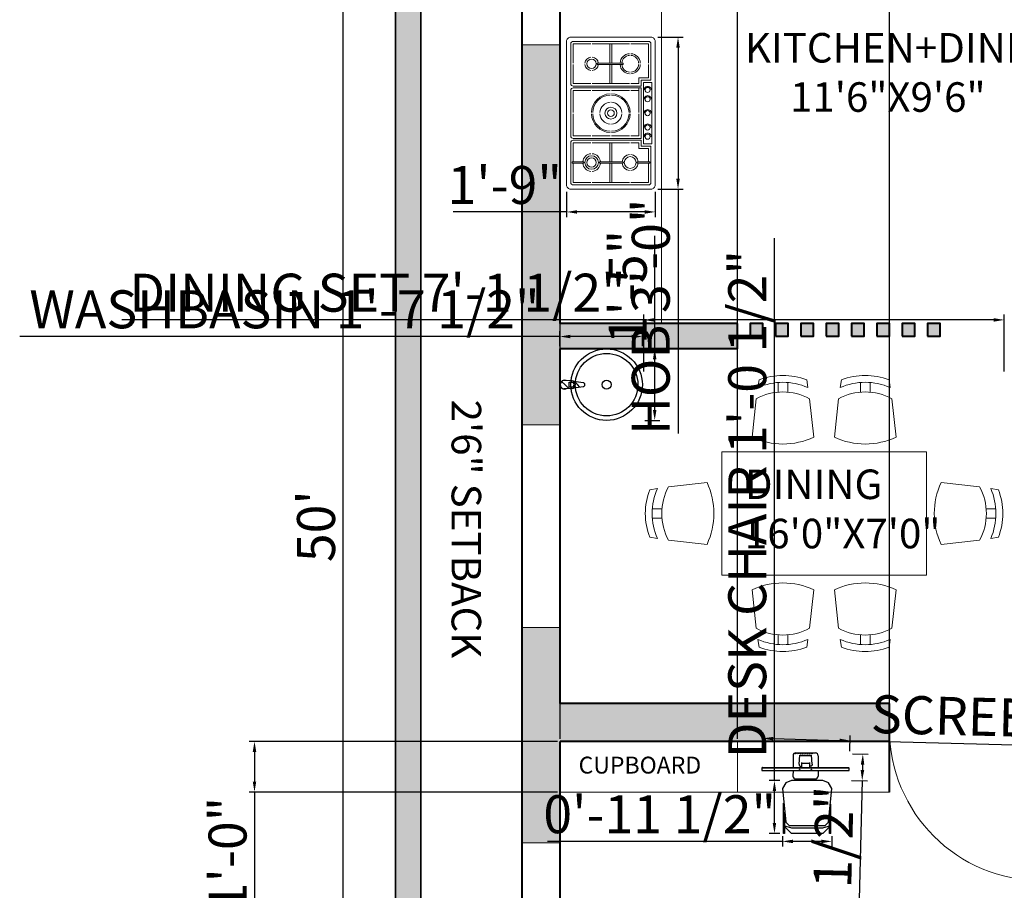
# Model space of a CAD drawing. Units: inches. Extents: x 2337 to 3570, y 1258 to 1938.
# Tile 3 of 30: x 2337 to 2570, y 1507 to 1713. Entities that reach past the tile are written whole.
import ezdxf

# ---------------------------------------------------------------- set-up
doc = ezdxf.new("R2010")
doc.units = ezdxf.units.IN
for name, color, linetype, lineweight in [('A-ANNO-DIMS', 2, 'Continuous', 18), ('A-ANNO-TEXT', 7, 'Continuous', 18), ('A-AREA-IDEN', 7, 'Continuous', 18), ('A-DOOR', 4, 'Continuous', 20), ('A-EQPM', 9, 'Continuous', 18), ('A-FLOR-CASE', 34, 'Continuous', 18), ('A-GLAZ', 4, 'Continuous', 18), ('A-WALL', 7, 'Continuous', 40), ('C-PROP', 7, 'Continuous', 35), ('furn', 8, 'Continuous', 18), ('Сантехника', 9, 'Continuous', 18)]:
    doc.layers.add(name, color=color, linetype=linetype, lineweight=lineweight)
doc.layers.add('A-WALL-PATT', color=18, linetype='Continuous', lineweight=13, true_color=0x000000)
doc.layers.add('C-PROP-PATT', color=251, linetype='Continuous', lineweight=13, true_color=0x636466)
for name, color, linetype in [('NOITHAT', 21, 'Continuous'), ('SANTEH', 7, 'Continuous'), ('window', 130, 'Continuous')]:
    doc.layers.add(name, color=color, linetype=linetype)
doc.styles.get("Standard").update_dxf_attribs({"font": 'arial.ttf'})
doc.dimstyles.new('ISO-25', dxfattribs={"dimtxt": 9, "dimasz": 2.5, "dimexe": 1.25, "dimexo": 0.625, "dimtad": 1, "dimdec": 1, "dimlunit": 3, "dimtxsty": 'Standard', "dimcen": 2.5, "dimadec": 0, "dimazin": 0, "dimtfac": 1, "dimtdec": 1, "dimtmove": 0, "dimatfit": 3, "dimfxl": 1, "dimarcsym": 0})
pattern_1 = [(45, (-0.056, -259.036), (-35.355, 35.355), [])]

# ---------------------------------------------------------------- blocks, each defined once
blk = doc.blocks.new('*U2')
for p, q in [((0, 0), (0, -6)), ((36, 0), (36, -6))]:
    blk.add_line(p, q)
blk.add_lwpolyline([(0, 0), (0, 36), (1.75, 36), (1.75, 0)], close=True)
blk.add_arc((0, 0), 36, 0, 90)
blk = doc.blocks.new('*D7')
at = {"layer": 'A-ANNO-DIMS', "color": 0, "lineweight": -2, "transparency": 16777216}
for p, q in [((2425.21, 1893.12), (2412.15, 1893.12)), ((2413.4, 1890.62), (2413.4, 1295.62)), ((2425.21, 1293.12), (2412.15, 1293.12))]:
    blk.add_line(p, q, dxfattribs=at)
at = {"layer": 'A-ANNO-DIMS', "color": 0, "transparency": 16777216}
for points in [[(2412.98, 1890.62), (2413.81, 1890.62), (2413.4, 1893.12)], [(2412.98, 1295.62), (2413.81, 1295.62), (2413.4, 1293.12)]]:
    blk.add_solid(points, dxfattribs=at)
at = {"layer": 'Defpoints', "color": 0, "transparency": 16777216}
for p in [(2425.84, 1893.12), (2413.4, 1293.12), (2425.84, 1293.12)]:
    blk.add_point(p, dxfattribs=at)
at = {"layer": 'A-ANNO-DIMS', "color": 0, "transparency": 16777216, "insert": (2408.18, 1593.12), "char_height": 9, "attachment_point": 5, "rotation": 90}
blk.add_mtext("50'", dxfattribs=at)
blk = doc.blocks.new('table-23')
at = {"color": 0, "linetype": 'ByBlock'}
for p, q in [((-0.6323, 0.4685), (-0.6236, 0.5245)), ((-0.485, 0.5057), (-0.485, 0.4355)), ((-0.415, 0.5057), (-0.415, 0.4355)), ((-0.2677, 0.4685), (-0.2764, 0.5245)), ((-0.675, 0.107), (-0.645, 0.387)), ((-0.225, 0.107), (-0.255, 0.387)), ((-0.9, -1.4923), (-0.9, 0)), ((-0.9, 0), (0, 0)), ((0, -1.4923), (0, 0)), ((-1.3677, -0.2639), (-1.4237, -0.2726)), ((-1.0062, -0.2211), (-1.2862, -0.2511)), ((0.1062, -0.2211), (0.3862, -0.2511)), ((0.4677, -0.2639), (0.5237, -0.2726)), ((-1.4049, -0.4111), (-1.3347, -0.4111)), ((0.5049, -0.4111), (0.4347, -0.4111)), ((-1.4049, -0.4811), (-1.3347, -0.4811)), ((0.5049, -0.4811), (0.4347, -0.4811)), ((-1.3677, -0.6284), (-1.4237, -0.6197)), ((-1.0062, -0.6711), (-1.2862, -0.6411)), ((0.1062, -0.6711), (0.3862, -0.6411)), ((0.4677, -0.6284), (0.5237, -0.6197)), ((-1.0062, -0.8211), (-1.2862, -0.8511)), ((0.1062, -0.8211), (0.3862, -0.8511)), ((-1.3677, -0.8639), (-1.4237, -0.8726)), ((0.4677, -0.8639), (0.5237, -0.8726)), ((-1.4049, -1.0111), (-1.3347, -1.0111)), ((0.5049, -1.0111), (0.4347, -1.0111)), ((-1.4049, -1.0811), (-1.3347, -1.0811)), ((0.5049, -1.0811), (0.4347, -1.0811)), ((-1.3677, -1.2284), (-1.4237, -1.2197)), ((0.4677, -1.2284), (0.5237, -1.2197)), ((-1.0062, -1.2711), (-1.2862, -1.2411)), ((0.1062, -1.2711), (0.3862, -1.2411)), ((-0.9, -1.4923), (0, -1.4923)), ((-0.675, -1.5993), (-0.645, -1.8793)), ((-0.225, -1.5993), (-0.255, -1.8793)), ((-0.485, -1.998), (-0.485, -1.9278)), ((-0.415, -1.998), (-0.415, -1.9278)), ((-0.6323, -1.9608), (-0.6236, -2.0168)), ((-0.2677, -1.9608), (-0.2764, -2.0168))]:
    blk.add_line(p, q, dxfattribs=at)
for centre, radius, start, end in [((-0.45, 0.0566), 0.4505, 66.13443, 113.86557), ((-0.45, 0.0773), 0.4797, 68.78869, 111.21131), ((-0.45, 0.0318), 0.4053, 61.23721, 118.76279), ((-0.45, 0.5883), 0.5312, 244.94238, 295.05762), ((-0.9765, -0.4461), 0.4797, 158.78869, 201.21131), ((-0.9558, -0.4461), 0.4505, 156.13443, 203.86557), ((-0.931, -0.4461), 0.4053, 151.23721, 208.76279), ((-1.4875, -0.4461), 0.5312, 334.94238, 25.05762), ((0.5875, -0.4461), 0.5312, 154.94238, 205.05762), ((0.031, -0.4461), 0.4053, 331.23721, 28.76279), ((0.0558, -0.4461), 0.4505, 336.13443, 23.86557), ((0.0765, -0.4461), 0.4797, 338.78869, 21.21131), ((-0.931, -1.0461), 0.4053, 151.23721, 208.76279), ((-1.4875, -1.0461), 0.5312, 334.94238, 25.05762), ((0.5875, -1.0461), 0.5312, 154.94238, 205.05762), ((0.031, -1.0461), 0.4053, 331.23721, 28.76279), ((-0.9765, -1.0461), 0.4797, 158.78869, 201.21131), ((-0.9558, -1.0461), 0.4505, 156.13443, 203.86557), ((0.0558, -1.0461), 0.4505, 336.13443, 23.86557), ((0.0765, -1.0461), 0.4797, 338.78869, 21.21131), ((-0.45, -2.0806), 0.5312, 64.94238, 115.05762), ((-0.45, -1.5241), 0.4053, 241.23721, 298.76279), ((-0.45, -1.5489), 0.4505, 246.13443, 293.86557), ((-0.45, -1.5696), 0.4797, 248.78869, 291.21131)]:
    blk.add_arc(centre, radius, start, end, dxfattribs=at)
blk = doc.blocks.new('STOVE')
for p, q in [((11.85, 19.7), (11.55, 19.7)), ((11.55, 16.92), (11.55, 19.7)), ((11.85, 16.92), (11.85, 19.7)), ((11.85, 16.92), (11.55, 16.92)), ((-11.85, 13.73), (-11.85, 7.62)), ((-11.85, 13.73), (-11.55, 13.73)), ((-11.55, 13.73), (-11.55, 7.62)), ((11.85, 13.23), (11.55, 13.23)), ((11.55, 13.23), (11.55, 7.57)), ((11.85, 13.23), (11.85, 7.57)), ((-11.85, 10.75), (-16.4, 10.75)), ((-11.85, 10.25), (-16.4, 10.25)), ((-7, 10.75), (-11.55, 10.75)), ((-7, 10.25), (-11.55, 10.25)), ((7, 10.75), (11.55, 10.75)), ((7, 10.25), (11.55, 10.25)), ((11.85, 10.75), (16.4, 10.75)), ((11.85, 10.25), (16.4, 10.25)), ((-11.85, 7.62), (-11.55, 7.62)), ((11.85, 7.57), (11.55, 7.57)), ((-7, 3.9), (-8.4, 3.9)), ((-7.8, 3.3), (-7.8, 1)), ((-6.4, 3.3), (-7.8, 3.3)), ((7.3, 2.8), (-7.3, 2.8)), ((-7.3, 2.8), (-7.3, 0.8)), ((-5.4, 3.9), (-6, 3.9)), ((-5.4, 3.9), (-0.15, 3.9)), ((0.15, 3.9), (5.4, 3.9)), ((6.4, 3.3), (7.8, 3.3)), ((7, 3.9), (8.4, 3.9)), ((7.3, 2.8), (7.3, 0.8)), ((7.8, 3.3), (7.8, 1)), ((8.4, 3.9), (8.4, 1.6)), ((11.85, 4.28), (11.55, 4.28)), ((11.55, 4.28), (11.55, 1.3)), ((11.85, 4.28), (11.85, 1.3)), ((7.3, 0.8), (-7.3, 0.8)), ((11.85, 1.3), (11.55, 1.3))]:
    blk.add_line(p, q)
for points in [[(-17, 21), (17, 21, -0.414214), (18, 20), (18, 1, -0.414214), (17, 0), (-17, 0, -0.414214), (-18, 1), (-18, 20, -0.414214)], [(6, 3.3), (-6, 3.3), (-6, 19.4, -0.414214), (-5.4, 20), (5.4, 20, -0.414214), (6, 19.4)]]:
    blk.add_lwpolyline(points, format="xyb", close=True)
for points in [[(-7.8, 1), (-16.4, 1, -0.414214), (-17, 1.6), (-17, 19.4, -0.414214), (-16.4, 20), (-7, 20, -0.414214), (-6.4, 19.4), (-6.4, 3.3)], [(6.4, 19.4, -0.414214), (7, 20), (16.4, 20, -0.414214), (17, 19.4), (17, 1.6, -0.414214), (16.4, 1), (7.8, 1)]]:
    blk.add_lwpolyline(points, format="xyb")
for points in [[(-16.4, 15.22), (-16.4, 19.4), (-11.85, 19.4)], [(-11.55, 19.4), (-7, 19.4), (-7, 15.22)], [(-5.4, 15.22), (-5.4, 19.4), (-0.15, 19.4)], [(0.15, 19.4), (5.4, 19.4), (5.4, 15.22)], [(6.4, 3.3), (6.4, 19.4)], [(7, 15.22), (7, 19.4), (11.55, 19.4)], [(11.85, 19.4), (16.4, 19.4), (16.4, 15.22)], [(-16.4, 6.08), (-16.4, 14.92)], [(-7, 14.92), (-7, 6.08)], [(-5.4, 10.65), (-5.4, 14.92)], [(5.4, 14.92), (5.4, 10.65)], [(7, 6.08), (7, 14.92)], [(16.4, 14.92), (16.4, 6.08)], [(-5.4, 6.08), (-5.4, 10.35)], [(5.4, 10.35), (5.4, 6.08)], [(-11.85, 1.6), (-16.4, 1.6), (-16.4, 5.77)], [(-7, 5.77), (-7, 3.9)], [(-5.4, 3.9), (-5.4, 5.77)], [(5.4, 5.77), (5.4, 3.9)], [(7, 3.9), (7, 5.77)], [(16.4, 5.77), (16.4, 1.6), (11.85, 1.6)], [(-8.4, 3.9), (-8.4, 1.6), (-11.55, 1.6)], [(11.55, 1.6), (8.4, 1.6)]]:
    blk.add_lwpolyline(points)
for centre, radius in [((11.7, 15.07), 1.6), ((-11.7, 15.07), 1.1), ((11.7, 15.07), 1.1), ((0, 10.5), 1.4), ((0, 10.5), 0.8), ((11.7, 5.93), 1.4), ((-5.49, 1.8), 0.6), ((-3.3, 1.8), 0.6), ((0, 1.8), 0.6), ((3.39, 1.8), 0.6), ((5.57, 1.8), 0.6)]:
    blk.add_circle(centre, radius)
for centre, radius, start, end in [((-11.7, 15.07), 1.6, 95.3794, 174.6206), ((-11.7, 15.07), 1.6, 5.3794, 84.6206), ((11.7, 15.07), 2.1, 94.096, 175.904), ((11.7, 15.07), 2.1, 4.096, 85.904), ((-11.7, 15.07), 1.6, 185.3794, 264.6206), ((-11.7, 15.07), 1.6, 275.3794, 354.6206), ((0, 10.5), 4.6, 91.8687, 178.1313), ((0, 10.5), 4.3, 91.9991, 178.0009), ((0, 10.5), 4.6, 1.8687, 88.1313), ((0, 10.5), 4.3, 1.9991, 88.0009), ((11.7, 15.07), 2.1, 184.096, 265.904), ((11.7, 15.07), 2.1, 274.096, 355.904), ((0, 10.5), 2.6, 93.3074, 176.6926), ((0, 10.5), 2.6, 3.3074, 86.6926), ((0, 10.5), 4.6, 181.8687, 268.1313), ((0, 10.5), 4.3, 181.9991, 268.0009), ((0, 10.5), 2.6, 183.3074, 266.6926), ((0, 10.5), 4.6, 271.8687, 358.1313), ((0, 10.5), 4.3, 271.9991, 358.0009), ((0, 10.5), 2.6, 273.3074, 356.6926), ((-11.7, 5.93), 2.4, 93.5833, 176.4167), ((-11.7, 5.93), 2, 94.3012, 175.6988), ((-11.7, 5.93), 2.4, 3.5833, 86.4167), ((-11.7, 5.93), 2, 4.3012, 85.6988), ((11.7, 5.93), 1.9, 94.5281, 175.4719), ((11.7, 5.93), 1.9, 4.5281, 85.4719), ((-11.7, 5.93), 2.4, 183.5833, 266.4167), ((-11.7, 5.93), 2, 184.3012, 265.6988), ((-11.7, 5.93), 2.4, 273.5833, 356.4167), ((-11.7, 5.93), 2, 274.3012, 355.6988), ((11.7, 5.93), 1.9, 184.5281, 265.4719), ((11.7, 5.93), 1.9, 274.5281, 355.4719), ((-5.49, 1.8), 0.846, 89.9979, 270), ((-3.3, 1.8), 0.846, 89.9979, 270), ((0, 1.8), 0.846, 89.9979, 270), ((3.39, 1.8), 0.846, 89.9979, 270), ((5.57, 1.8), 0.846, 89.9979, 270)]:
    blk.add_arc(centre, radius, start, end)
blk = doc.blocks.new('TV')
at = {"color": 0}
for p, q in [((3967.27, 1784.85), (3967.05, 1784.65)), ((3967.76, 1763.68), (3967.54, 1763.86))]:
    blk.add_line(p, q, dxfattribs=at)
at = {"layer": 'window'}
for p, q in [((3967.54, 1763.86), (3967.05, 1784.65)), ((3964.41, 1777.23), (3967.22, 1777.3)), ((3968.01, 1777.32), (3969.36, 1777.35)), ((3966.53, 1775.82), (3964.33, 1775.61)), ((3964.34, 1775.34), (3964.45, 1775.34)), ((3964.34, 1775.31), (3964.43, 1775.32)), ((3966.14, 1775.2), (3967.01, 1775.22)), ((3966.14, 1775.18), (3967.27, 1775.2)), ((3966.14, 1775.18), (3966.14, 1775.2)), ((3966.3, 1773.29), (3966.26, 1775.18)), ((3964.39, 1773.06), (3964.48, 1773.06)), ((3964.39, 1773.04), (3964.5, 1773.04)), ((3966.61, 1772.66), (3964.4, 1772.77)), ((3966.19, 1773.28), (3967.31, 1773.31)), ((3966.19, 1773.26), (3967.05, 1773.28)), ((3966.19, 1773.26), (3966.19, 1773.28)), ((3964.55, 1771.15), (3967.36, 1771.22)), ((3968.15, 1771.24), (3969.5, 1771.27))]:
    blk.add_line(p, q, dxfattribs=at)
for points in [[(3968.33, 1763.69), (3967.83, 1784.86), (3967.27, 1784.85), (3967.76, 1763.68), (3968.33, 1763.69)], [(3963.86, 1771.81), (3963.75, 1776.54)], [(3970.16, 1771.96), (3970.05, 1776.69)], [(3964.4, 1772.77), (3964.33, 1775.61)], [(3964.48, 1773.06), (3964.43, 1775.32)], [(3964.5, 1773.04), (3964.45, 1775.34)]]:
    blk.add_lwpolyline(points, dxfattribs=at)
for points in [[(3966.53, 1775.82, -0.263666), (3966.93, 1775.69), (3967, 1775.57), (3967.01, 1775.22)], [(3966.61, 1772.66, 0.263666), (3967, 1772.81), (3967.06, 1772.93), (3967.05, 1773.28)]]:
    blk.add_lwpolyline(points, format="xyb", dxfattribs=at)
for centre, radius in [((3963.91, 1775.73), 0.0679), ((3963.93, 1775.17), 0.0679), ((3963.94, 1774.6), 0.0679), ((3963.95, 1774.04), 0.0679), ((3967.77, 1775.68), 0.0451), ((3963.97, 1773.48), 0.0679), ((3963.98, 1772.92), 0.0679), ((3963.99, 1772.35), 0.0679), ((3964.01, 1771.79), 0.0679), ((3967.83, 1772.86), 0.0451)]:
    blk.add_circle(centre, radius, dxfattribs=at)
for centre, start, end in [((3964.42, 1776.56), 91.3414, 181.3414), ((3969.38, 1776.67), 1.3414, 91.3414), ((3964.53, 1771.83), 181.3414, 271.3414), ((3969.49, 1771.94), 271.3414, 1.3414)]:
    blk.add_arc(centre, 0.676, start, end, dxfattribs=at)
blk = doc.blocks.new('A$C702B4F5C')
at = {"layer": 'NOITHAT'}
blk.add_lwpolyline([(78.8, 67.5), (112.5, 33.8), (450, 0), (506.3, 33.8), (528.8, 90), (528.8, 405), (506.3, 461.3), (450, 495), (112.5, 461.3), (78.8, 427.5)], close=True, dxfattribs=at)
for points in [[(78.8, 483.8), (56.3, 405), (56.3, 90), (78.8, 11.3), (0, 90), (0, 405), (78.8, 483.8)], [(67.5, 472.5), (0, 472.5), (0, 483.8), (303.8, 483.8)], [(213.8, 472.5), (78.8, 472.5)], [(0, 11.3), (0, 22.5), (67.5, 22.5)], [(0, 11.3), (292.5, 11.3)], [(78.8, 22.5), (213.8, 22.5)]]:
    blk.add_lwpolyline(points, dxfattribs=at)
blk = doc.blocks.new('r13')
at = {"layer": 'SANTEH', "ltscale": 5}
h = blk.add_hatch(dxfattribs=at)
h.set_pattern_fill('100__1', color=256, scale=0.5, angle=45, style=0)
h.set_pattern_definition(pattern_1)
h.paths.add_polyline_path([(-0.1, -138.2, -0.378173), (-11.2, -128.4), (-17.8, -75.5, -0.12102), (-21.1, -66), (-23.4, -32.9, -0.524536), (-0.1, 1)], flags=0)
h = blk.add_hatch(dxfattribs=at)
h.set_pattern_fill('100__1', color=256, scale=0.5, angle=45, style=0)
h.set_pattern_definition(pattern_1)
h.paths.add_polyline_path([(-0.1, -138.2, 0.378173), (11, -128.4), (17.7, -75.5, 0.12102), (20.9, -66), (23.3, -32.9, 0.524536), (-0.1, 1)], flags=0)
for p, q in [((-24, -25.7), (-23.9, -20.6)), ((-21.1, -66), (-24, -25.7)), ((-13.7, -48.9), (13.5, -48.9)), ((-13.7, -63.8), (-13.7, -48.9)), ((-13.7, -49.6), (13.5, -49.6)), ((13.5, -48.9), (13.5, -63.8)), ((20.9, -66), (23.8, -25.7)), ((23.8, -25.7), (23.8, -20.7)), ((-17.8, -75.5), (-11.2, -128.4)), ((11, -128.4), (17.7, -75.5))]:
    blk.add_line(p, q, dxfattribs=at)
for radius in [200, 175, 25]:
    blk.add_circle((-0.1, -259), radius, dxfattribs=at)
for centre, radius, start, end in [((-0.1, -24), 25, 339.2856, 200.7144), ((-0.1, -24), 24, 7.8374, 171.8967), ((-0.1, -63.4), 21.1, 185.1696, 354.8304), ((-0.1, -64.1), 21.1, 185.1696, 354.8304), ((-0.1, -63.8), 13.6, 180, 0), ((-0.1, -127), 11.2, 187.1389, 352.8611)]:
    blk.add_arc(centre, radius, start, end, dxfattribs=at)
blk = doc.blocks.new('SCREEN-DIVIDER-8-POST')
h = blk.add_hatch(color=256)
h.dxf.hatch_style = 1
h.paths.add_polyline_path([(3, 3), (0, 3), (0, 0), (3, 0)])
h = blk.add_hatch(color=256)
h.dxf.hatch_style = 1
h.paths.add_polyline_path([(6, 3), (6, 0), (9, 0), (9, 3)])
h = blk.add_hatch(color=256)
h.dxf.hatch_style = 1
h.paths.add_polyline_path([(15, 3), (12, 3), (12, 0), (15, 0)])
h = blk.add_hatch(color=256)
h.dxf.hatch_style = 1
h.paths.add_polyline_path([(18, 3), (18, 0), (21, 0), (21, 3)])
h = blk.add_hatch(color=256)
h.dxf.hatch_style = 1
h.paths.add_polyline_path([(27, 3), (24, 3), (24, 0), (27, 0)])
h = blk.add_hatch(color=256)
h.dxf.hatch_style = 1
h.paths.add_polyline_path([(30, 3), (30, 0), (33, 0), (33, 3)])
h = blk.add_hatch(color=256)
h.dxf.hatch_style = 1
h.paths.add_polyline_path([(39, 3), (36, 3), (36, 0), (39, 0)])
h = blk.add_hatch(color=256)
h.dxf.hatch_style = 1
h.paths.add_polyline_path([(42, 3), (42, 0), (45, 0), (45, 3)])
for points in [[(0, 0), (3, 0), (3, 3), (0, 3)], [(6, 0), (9, 0), (9, 3), (6, 3)], [(12, 0), (15, 0), (15, 3), (12, 3)], [(18, 0), (21, 0), (21, 3), (18, 3)], [(24, 0), (27, 0), (27, 3), (24, 3)], [(30, 0), (33, 0), (33, 3), (30, 3)], [(36, 0), (39, 0), (39, 3), (36, 3)], [(42, 0), (45, 0), (45, 3), (42, 3)]]:
    blk.add_lwpolyline(points, close=True)
blk = doc.blocks.new('*D56')
at = {"layer": 'A-ANNO-DIMS', "color": 0, "lineweight": -2, "transparency": 16777216}
for p, q in [((2512.75, 1540.36), (2512.84, 1544.09)), ((2515.31, 1542.78), (2531.03, 1542.38)), ((2533.46, 1539.83), (2533.56, 1543.56)), ((2533.53, 1542.31), (2637.99, 1539.66))]:
    blk.add_line(p, q, dxfattribs=at)
at = {"layer": 'A-ANNO-DIMS', "color": 0, "transparency": 16777216}
for points in [[(2515.32, 1543.19), (2515.3, 1542.36), (2512.81, 1542.84)], [(2531.04, 1542.79), (2531.02, 1541.96), (2533.53, 1542.31)]]:
    blk.add_solid(points, dxfattribs=at)
at = {"layer": 'Defpoints', "color": 0, "transparency": 16777216}
for p in [(2533.53, 1542.31), (2512.73, 1539.73), (2533.45, 1539.2)]:
    blk.add_point(p, dxfattribs=at)
at = {"layer": 'A-ANNO-DIMS', "color": 0, "transparency": 16777216, "insert": (2587.14, 1546.23), "char_height": 9, "attachment_point": 5, "rotation": 358.5431}
blk.add_mtext('SCREEN 1\'-8 1/2"', dxfattribs=at)
blk = doc.blocks.new('*D57')
at = {"layer": 'A-ANNO-DIMS', "color": 0, "lineweight": -2, "transparency": 16777216}
for p, q in [((2534.07, 1539.19), (2537.81, 1539.09)), ((2536.49, 1536.63), (2536.46, 1535.34)), ((2533.91, 1532.9), (2537.65, 1532.81)), ((2536.4, 1532.84), (2535.16, 1484.21))]:
    blk.add_line(p, q, dxfattribs=at)
at = {"layer": 'A-ANNO-DIMS', "color": 0, "transparency": 16777216}
for points in [[(2536.08, 1536.64), (2536.91, 1536.62), (2536.56, 1539.13)], [(2536.04, 1535.35), (2536.88, 1535.33), (2536.4, 1532.84)]]:
    blk.add_solid(points, dxfattribs=at)
at = {"layer": 'Defpoints', "color": 0, "transparency": 16777216}
for p in [(2533.45, 1539.2), (2533.29, 1532.92), (2536.4, 1532.84)]:
    blk.add_point(p, dxfattribs=at)
at = {"layer": 'A-ANNO-DIMS', "color": 0, "transparency": 16777216, "insert": (2530.47, 1507.41), "char_height": 9, "attachment_point": 5, "rotation": 88.5431}
blk.add_mtext('0\'-6 1/2"', dxfattribs=at)
blk = doc.blocks.new('*D78')
at = {"layer": 'A-ANNO-DIMS', "color": 0, "lineweight": -2, "transparency": 16777216}
for p, q in [((2484.66, 1629.8), (2484.66, 1643.24)), ((2570.07, 1629.8), (2570.07, 1643.24)), ((2484.66, 1641.99), (2361.02, 1641.99)), ((2567.57, 1641.99), (2487.16, 1641.99))]:
    blk.add_line(p, q, dxfattribs=at)
at = {"layer": 'A-ANNO-DIMS', "color": 0, "transparency": 16777216}
for points in [[(2487.16, 1642.4), (2487.16, 1641.57), (2484.66, 1641.99)], [(2567.57, 1642.4), (2567.57, 1641.57), (2570.07, 1641.99)]]:
    blk.add_solid(points, dxfattribs=at)
at = {"layer": 'Defpoints', "color": 0, "transparency": 16777216}
for p in [(2484.66, 1641.99), (2484.66, 1629.18), (2570.07, 1629.18)]:
    blk.add_point(p, dxfattribs=at)
at = {"layer": 'A-ANNO-DIMS', "color": 0, "transparency": 16777216, "insert": (2421.59, 1647.27), "char_height": 9, "attachment_point": 5}
blk.add_mtext('DINING SET 7\'-1 1/2"', dxfattribs=at)
blk = doc.blocks.new('*D82')
at = {"layer": 'A-ANNO-DIMS', "color": 0, "lineweight": -2, "transparency": 16777216}
for p, q in [((2487.99, 1708.97), (2494.02, 1708.97)), ((2492.77, 1706.47), (2492.77, 1675.47)), ((2487.99, 1672.97), (2494.02, 1672.97)), ((2492.77, 1672.97), (2492.77, 1615.04))]:
    blk.add_line(p, q, dxfattribs=at)
at = {"layer": 'A-ANNO-DIMS', "color": 0, "transparency": 16777216}
for points in [[(2492.35, 1706.47), (2493.19, 1706.47), (2492.77, 1708.97)], [(2492.35, 1675.47), (2493.19, 1675.47), (2492.77, 1672.97)]]:
    blk.add_solid(points, dxfattribs=at)
at = {"layer": 'Defpoints', "color": 0, "transparency": 16777216}
for p in [(2487.37, 1708.97), (2487.37, 1672.97), (2492.77, 1672.97)]:
    blk.add_point(p, dxfattribs=at)
at = {"layer": 'A-ANNO-DIMS', "color": 0, "transparency": 16777216, "insert": (2487.48, 1642.75), "char_height": 9, "attachment_point": 5, "rotation": 90}
blk.add_mtext('HOB 3\'-0"', dxfattribs=at)
blk = doc.blocks.new('*D83')
at = {"layer": 'A-ANNO-DIMS', "color": 0, "lineweight": -2, "transparency": 16777216}
for p, q in [((2466.37, 1672.34), (2466.37, 1666.32)), ((2487.37, 1672.34), (2487.37, 1666.32)), ((2466.37, 1667.57), (2439.54, 1667.57)), ((2484.87, 1667.57), (2468.87, 1667.57))]:
    blk.add_line(p, q, dxfattribs=at)
at = {"layer": 'A-ANNO-DIMS', "color": 0, "transparency": 16777216}
for points in [[(2468.87, 1667.98), (2468.87, 1667.15), (2466.37, 1667.57)], [(2484.87, 1667.98), (2484.87, 1667.15), (2487.37, 1667.57)]]:
    blk.add_solid(points, dxfattribs=at)
at = {"layer": 'Defpoints', "color": 0, "transparency": 16777216}
for p in [(2466.37, 1672.97), (2487.37, 1672.97), (2466.37, 1667.57)]:
    blk.add_point(p, dxfattribs=at)
at = {"layer": 'A-ANNO-DIMS', "color": 0, "transparency": 16777216, "insert": (2451.71, 1672.79), "char_height": 9, "attachment_point": 5}
blk.add_mtext('1\'-9"', dxfattribs=at)
blk = doc.blocks.new('*D92')
at = {"layer": 'A-ANNO-DIMS', "color": 0, "lineweight": -2, "transparency": 16777216}
for p, q in [((2515.62, 1532.84), (2515.62, 1661.38)), ((2516.87, 1532.84), (2514.37, 1532.84)), ((2515.62, 1522.81), (2515.62, 1530.34)), ((2516.87, 1520.31), (2514.37, 1520.31))]:
    blk.add_line(p, q, dxfattribs=at)
at = {"layer": 'A-ANNO-DIMS', "color": 0, "transparency": 16777216}
for points in [[(2515.2, 1530.34), (2516.03, 1530.34), (2515.62, 1532.84)], [(2515.2, 1522.81), (2516.03, 1522.81), (2515.62, 1520.31)]]:
    blk.add_solid(points, dxfattribs=at)
at = {"layer": 'Defpoints', "color": 0, "transparency": 16777216}
for p in [(2515.62, 1532.84), (2517.5, 1532.84), (2517.5, 1520.31)]:
    blk.add_point(p, dxfattribs=at)
at = {"layer": 'A-ANNO-DIMS', "color": 0, "transparency": 16777216, "insert": (2510.34, 1598.36), "char_height": 9, "attachment_point": 5, "rotation": 90}
blk.add_mtext('DESK CHAIR 1\'-0 1/2"', dxfattribs=at)
blk = doc.blocks.new('*D93')
at = {"layer": 'A-ANNO-DIMS', "color": 0, "lineweight": -2, "transparency": 16777216}
for p, q in [((2517.5, 1519.69), (2517.5, 1517.19)), ((2529.22, 1519.69), (2529.22, 1517.19)), ((2517.5, 1518.44), (2461.86, 1518.44)), ((2526.72, 1518.44), (2520, 1518.44))]:
    blk.add_line(p, q, dxfattribs=at)
at = {"layer": 'A-ANNO-DIMS', "color": 0, "transparency": 16777216}
for points in [[(2520, 1518.85), (2520, 1518.02), (2517.5, 1518.44)], [(2526.72, 1518.85), (2526.72, 1518.02), (2529.22, 1518.44)]]:
    blk.add_solid(points, dxfattribs=at)
at = {"layer": 'Defpoints', "color": 0, "transparency": 16777216}
for p in [(2517.5, 1520.31), (2529.22, 1520.31), (2517.5, 1518.44)]:
    blk.add_point(p, dxfattribs=at)
at = {"layer": 'A-ANNO-DIMS', "color": 0, "transparency": 16777216, "insert": (2488.43, 1523.71), "char_height": 9, "attachment_point": 5}
blk.add_mtext('0\'-11 1/2"', dxfattribs=at)
blk = doc.blocks.new('*D94')
at = {"layer": 'A-ANNO-DIMS', "color": 0, "lineweight": -2, "transparency": 16777216}
for p, q in [((2464.77, 1638.05), (2336.81, 1638.05)), ((2464.77, 1635.74), (2464.77, 1639.3)), ((2481.82, 1638.05), (2467.27, 1638.05)), ((2484.32, 1635.74), (2484.32, 1639.3))]:
    blk.add_line(p, q, dxfattribs=at)
at = {"layer": 'A-ANNO-DIMS', "color": 0, "transparency": 16777216}
for points in [[(2467.27, 1638.47), (2467.27, 1637.63), (2464.77, 1638.05)], [(2481.82, 1638.47), (2481.82, 1637.63), (2484.32, 1638.05)]]:
    blk.add_solid(points, dxfattribs=at)
at = {"layer": 'Defpoints', "color": 0, "transparency": 16777216}
for p in [(2464.77, 1638.05), (2464.77, 1635.12), (2484.32, 1635.12)]:
    blk.add_point(p, dxfattribs=at)
at = {"layer": 'A-ANNO-DIMS', "color": 0, "transparency": 16777216, "insert": (2399.54, 1643.33), "char_height": 9, "attachment_point": 5}
blk.add_mtext('WASHBASIN 1\'-7 1/2"', dxfattribs=at)
blk = doc.blocks.new('*D95')
at = {"layer": 'A-ANNO-DIMS', "color": 0, "lineweight": -2, "transparency": 16777216}
for p, q in [((2487.25, 1635.12), (2487.25, 1661.94)), ((2484.94, 1635.12), (2488.5, 1635.12)), ((2487.25, 1620.68), (2487.25, 1632.62)), ((2484.94, 1618.18), (2488.5, 1618.18))]:
    blk.add_line(p, q, dxfattribs=at)
at = {"layer": 'A-ANNO-DIMS', "color": 0, "transparency": 16777216}
for points in [[(2486.83, 1632.62), (2487.67, 1632.62), (2487.25, 1635.12)], [(2486.83, 1620.68), (2487.67, 1620.68), (2487.25, 1618.18)]]:
    blk.add_solid(points, dxfattribs=at)
at = {"layer": 'Defpoints', "color": 0, "transparency": 16777216}
for p in [(2484.32, 1635.12), (2487.25, 1635.12), (2484.32, 1618.18)]:
    blk.add_point(p, dxfattribs=at)
at = {"layer": 'A-ANNO-DIMS', "color": 0, "transparency": 16777216, "insert": (2482.03, 1649.78), "char_height": 9, "attachment_point": 5, "rotation": 90}
blk.add_mtext('1\'-5"', dxfattribs=at)
blk = doc.blocks.new('*D106')
at = {"layer": 'A-ANNO-DIMS', "color": 0, "lineweight": -2, "transparency": 16777216}
for p, q in [((2464.84, 1542.74), (2464.84, 1927.77)), ((2506.84, 1542.74), (2506.84, 1927.77)), ((2467.34, 1926.52), (2504.34, 1926.52))]:
    blk.add_line(p, q, dxfattribs=at)
at = {"layer": 'A-ANNO-DIMS', "color": 0, "transparency": 16777216}
for points in [[(2467.34, 1926.93), (2467.34, 1926.1), (2464.84, 1926.52)], [(2504.34, 1926.93), (2504.34, 1926.1), (2506.84, 1926.52)]]:
    blk.add_solid(points, dxfattribs=at)
at = {"layer": 'Defpoints', "color": 0, "transparency": 16777216}
for p in [(2506.84, 1926.52), (2464.84, 1542.12), (2506.84, 1542.12)]:
    blk.add_point(p, dxfattribs=at)
at = {"layer": 'A-ANNO-DIMS', "color": 0, "transparency": 16777216, "insert": (2485.84, 1931.74), "char_height": 9, "attachment_point": 5}
blk.add_mtext('3\'-6"', dxfattribs=at)
blk = doc.blocks.new('*D107')
at = {"layer": 'A-ANNO-DIMS', "color": 0, "lineweight": -2, "transparency": 16777216}
for p, q in [((2506.84, 1542.74), (2506.84, 1927.77)), ((2542.84, 1542.74), (2542.84, 1927.77)), ((2509.34, 1926.52), (2540.34, 1926.52))]:
    blk.add_line(p, q, dxfattribs=at)
at = {"layer": 'A-ANNO-DIMS', "color": 0, "transparency": 16777216}
for points in [[(2509.34, 1926.93), (2509.34, 1926.1), (2506.84, 1926.52)], [(2540.34, 1926.93), (2540.34, 1926.1), (2542.84, 1926.52)]]:
    blk.add_solid(points, dxfattribs=at)
at = {"layer": 'Defpoints', "color": 0, "transparency": 16777216}
for p in [(2542.84, 1926.52), (2506.84, 1542.12), (2542.84, 1542.12)]:
    blk.add_point(p, dxfattribs=at)
at = {"layer": 'A-ANNO-DIMS', "color": 0, "transparency": 16777216, "insert": (2524.84, 1931.74), "char_height": 9, "attachment_point": 5}
blk.add_mtext('3\'-0"', dxfattribs=at)
blk = doc.blocks.new('*D108')
at = {"layer": 'A-ANNO-DIMS', "color": 0, "lineweight": -2, "transparency": 16777216}
for p, q in [((2464.21, 1542.12), (2391.19, 1542.12)), ((2392.44, 1539.62), (2392.44, 1532.62)), ((2464.21, 1530.12), (2391.19, 1530.12)), ((2392.44, 1530.12), (2392.44, 1503.29))]:
    blk.add_line(p, q, dxfattribs=at)
at = {"layer": 'A-ANNO-DIMS', "color": 0, "transparency": 16777216}
for points in [[(2392.02, 1539.62), (2392.85, 1539.62), (2392.44, 1542.12)], [(2392.02, 1532.62), (2392.85, 1532.62), (2392.44, 1530.12)]]:
    blk.add_solid(points, dxfattribs=at)
at = {"layer": 'Defpoints', "color": 0, "transparency": 16777216}
for p in [(2464.84, 1542.12), (2392.44, 1530.12), (2464.84, 1530.12)]:
    blk.add_point(p, dxfattribs=at)
at = {"layer": 'A-ANNO-DIMS', "color": 0, "transparency": 16777216, "insert": (2387.22, 1515.45), "char_height": 9, "attachment_point": 5, "rotation": 90}
blk.add_mtext('1\'-0"', dxfattribs=at)

msp = doc.modelspace()

# ---------------------------------------------------------------- hatches: boundary and pattern name
at = {"layer": 'A-WALL-PATT'}
h = msp.add_hatch(color=256, dxfattribs=at)
h.dxf.hatch_style = 1
h.paths.add_polyline_path([(2671.84, 1857.12), (2455.84, 1857.12), (2455.84, 1824.12), (2464.84, 1824.12), (2464.84, 1848.12), (2671.84, 1848.12)])
h.paths.add_polyline_path([(2566.84, 1764.12), (2464.84, 1764.12), (2464.84, 1788.12), (2455.84, 1788.12), (2455.84, 1743.12), (2464.84, 1743.12), (2464.84, 1755.12), (2566.84, 1755.12)])
h.paths.add_polyline_path([(2683.84, 1761.12), (2683.84, 1764.12), (2602.84, 1764.12), (2602.84, 1755.12), (2608.84, 1755.12), (2608.84, 1701.12), (2662.84, 1701.12), (2662.84, 1605.12), (2671.84, 1605.12), (2671.84, 1713.12), (2662.84, 1713.12), (2662.84, 1707.12), (2614.84, 1707.12), (2614.84, 1755.12), (2662.84, 1755.12), (2662.84, 1749.12), (2671.84, 1749.12), (2671.84, 1755.12), (2683.84, 1755.12)])
h.paths.add_polyline_path([(2464.84, 1707.12), (2455.84, 1707.12), (2455.84, 1617.12), (2464.84, 1617.12), (2464.84, 1635.12), (2506.84, 1635.12), (2506.84, 1641.12), (2464.84, 1641.12)])
h.paths.add_polyline_path([(2542.84, 1551.12), (2464.84, 1551.12), (2464.84, 1569.12), (2455.84, 1569.12), (2455.84, 1518.12), (2464.84, 1518.12), (2464.84, 1542.12), (2542.84, 1542.12)])
h.paths.add_polyline_path([(2464.84, 1482.12), (2455.84, 1482.12), (2455.84, 1410.12), (2464.84, 1410.12)])
h.paths.add_polyline_path([(2626.84, 1350.12), (2590.84, 1350.12), (2590.84, 1380.12), (2584.84, 1380.12), (2584.84, 1350.12), (2464.84, 1350.12), (2464.84, 1374.12), (2455.84, 1374.12), (2455.84, 1341.12), (2626.84, 1341.12)])
h.paths.add_polyline_path([(2662.84, 1416.12), (2686.84, 1416.12), (2686.84, 1422.12), (2590.84, 1422.12), (2590.84, 1542.12), (2680.84, 1542.12), (2680.84, 1551.12), (2671.84, 1551.12), (2671.84, 1557.12), (2662.84, 1557.12), (2662.84, 1551.12), (2578.84, 1551.12), (2578.84, 1542.12), (2584.84, 1542.12), (2584.84, 1410.12), (2590.84, 1410.12), (2590.84, 1416.12), (2656.84, 1416.12), (2656.84, 1350.12), (2650.84, 1350.12), (2650.84, 1341.12), (2731.84, 1341.12), (2731.84, 1362.12), (2722.84, 1362.12), (2722.84, 1350.12), (2662.84, 1350.12)])
h.paths.add_polyline_path([(2731.84, 1434.12), (2722.84, 1434.12), (2722.84, 1422.12), (2716.84, 1422.12), (2716.84, 1416.12), (2722.84, 1416.12), (2722.84, 1386.12), (2731.84, 1386.12)], flags=17)
h.paths.add_polyline_path([(2731.84, 1542.12), (2752.84, 1542.12), (2752.84, 1551.12), (2716.84, 1551.12), (2716.84, 1545.12), (2716.84, 1542.12), (2722.84, 1542.12), (2722.84, 1482.12), (2731.84, 1482.12)])
h.paths.add_polyline_path([(2809.84, 1551.12), (2788.84, 1551.12), (2788.84, 1542.12), (2809.84, 1542.12), (2809.84, 1548.12)])
h.paths.add_polyline_path([(2872.84, 1647.12), (2863.84, 1647.12), (2863.84, 1551.12), (2857.84, 1551.12), (2857.84, 1548.12), (2857.84, 1542.12), (2872.84, 1542.12)])
h.paths.add_polyline_path([(2872.84, 1764.12), (2827.84, 1764.12), (2827.84, 1755.12), (2863.84, 1755.12), (2863.84, 1719.12), (2872.84, 1719.12)])
h.paths.add_polyline_path([(2755.84, 1764.12), (2719.84, 1764.12), (2719.84, 1755.12), (2755.84, 1755.12)])
at = {"layer": 'C-PROP-PATT'}
h = msp.add_hatch(color=256, dxfattribs=at)
h.dxf.hatch_style = 1
h.paths.add_polyline_path([(2905.84, 1893.12), (2425.84, 1893.12), (2425.84, 1293.12), (2731.84, 1293.12), (2731.84, 1299.12), (2431.84, 1299.12), (2431.84, 1887.12), (2899.84, 1887.12), (2899.84, 1875.12), (2905.84, 1875.12)])
h.paths.add_polyline_path([(2845.84, 1299.12), (2827.84, 1299.12), (2827.84, 1293.12), (2845.84, 1293.12)], flags=17)
h.paths.add_polyline_path([(2905.84, 1779.12), (2899.84, 1779.12), (2899.84, 1299.12), (2893.84, 1299.12), (2893.84, 1293.12), (2905.84, 1293.12)], flags=17)

# ---------------------------------------------------------------- linework, layer by layer
at = {"layer": 'A-FLOR-CASE'}
for p, q in [((2488.84, 1641.12), (2488.84, 1731.12)), ((2506.84, 1530.12), (2506.84, 1542.12)), ((2542.84, 1530.12), (2464.84, 1530.12))]:
    msp.add_line(p, q, dxfattribs=at)
at = {"layer": 'A-GLAZ'}
for p, q in [((2464.84, 1707.12), (2455.84, 1707.12)), ((2464.84, 1617.12), (2455.84, 1617.12)), ((2464.84, 1569.12), (2455.84, 1569.12)), ((2464.84, 1518.12), (2455.84, 1518.12))]:
    msp.add_line(p, q, dxfattribs=at)
at = {"layer": 'A-WALL'}
for p, q in [((2455.84, 1341.12), (2455.84, 1857.12)), ((2464.84, 1641.12), (2464.84, 1755.12)), ((2506.84, 1641.12), (2464.84, 1641.12)), ((2506.84, 1635.12), (2506.84, 1641.12)), ((2506.84, 1635.12), (2464.84, 1635.12)), ((2464.84, 1551.12), (2464.84, 1635.12)), ((2542.84, 1551.12), (2464.84, 1551.12)), ((2542.84, 1530.12), (2542.84, 1551.12)), ((2542.84, 1542.12), (2464.84, 1542.12)), ((2464.84, 1350.12), (2464.84, 1542.12))]:
    msp.add_line(p, q, dxfattribs=at)
at = {"layer": 'C-PROP'}
for p, q in [((2425.84, 1293.12), (2425.84, 1893.12)), ((2431.84, 1299.12), (2431.84, 1887.12))]:
    msp.add_line(p, q, dxfattribs=at)

# ---------------------------------------------------------------- block references
at = {"layer": 'A-DOOR', "rotation": 180}
msp.add_blockref('*U2', (2578.84, 1545.12), dxfattribs=at)
at = {"layer": 'A-EQPM', "xscale": -1, "rotation": 90}
msp.add_blockref('STOVE', (2487.37, 1690.97), dxfattribs=at)
at = {"layer": 'A-EQPM', "xscale": 0.9782889442114187, "yscale": 0.9782889442114187, "zscale": 0.9782889442114187, "rotation": 268.5430845181614}
msp.add_blockref('TV', (886.49, 5460.03), dxfattribs=at)
at = {"layer": 'A-WALL'}
msp.add_blockref('SCREEN-DIVIDER-8-POST', (2509.84, 1638.12), dxfattribs=at)
at = {"layer": 'furn', "rotation": 90}
for name, p, xscale, yscale, zscale in [('table-23', (2503.12, 1610.75), 32.50065408352129, 32.50065408352129, 32.50065408352129), ('A$C702B4F5C', (2529.22, 1520.31), 0.0236823496324337, 0.0236823496324337, 0.0236823496324337)]:
    msp.add_blockref(name, p, dxfattribs=dict(at, xscale=xscale, yscale=yscale, zscale=zscale))
at = {"layer": 'Сантехника', "xscale": 0.0423505493012471, "yscale": 0.0423505493012471, "zscale": 0.0423505493012471, "rotation": 90}
msp.add_blockref('r13', (2464.88, 1626.65), dxfattribs=at)

# ---------------------------------------------------------------- texts
at = {"layer": 'A-ANNO-TEXT', "insert": (2446.13, 1623.11), "char_height": 7, "attachment_point": 1, "rotation": 270}
msp.add_mtext_dynamic_manual_height_columns('2\'6" SETBACK', width=66.911, gutter_width=12.5, heights=[0], dxfattribs=at)
at = {"layer": 'A-ANNO-TEXT', "insert": (2469.22, 1538.51), "char_height": 4, "attachment_point": 1}
msp.add_mtext_dynamic_manual_height_columns('CUPBOARD', width=66.911, gutter_width=12.5, heights=[0], dxfattribs=at)
at = {"layer": 'A-AREA-IDEN', "char_height": 7, "attachment_point": 1}
for s, insert in [('KITCHEN+DINING\\P     11\'6"X9\'6"', (2508.61, 1709.96)), ('DINING\\P16\'0"X7\'0"', (2508.61, 1606.54))]:
    msp.add_mtext_dynamic_manual_height_columns(s, width=66.911, gutter_width=12.5, heights=[0], dxfattribs=dict(at, insert=insert))

# ---------------------------------------------------------------- dimensions: what is measured, and where the dimension line sits
at = {"layer": 'A-ANNO-DIMS'}
for base, p1, p2, picture, middle in [((2506.84, 1926.52), (2464.84, 1542.12), (2506.84, 1542.12), '*D106', (2485.84, 1931.74)), ((2542.84, 1926.52), (2506.84, 1542.12), (2542.84, 1542.12), '*D107', (2524.84, 1931.74))]:
    dim = msp.add_linear_dim(base=base, p1=p1, p2=p2, dimstyle='ISO-25', override={"dimdec": 1, "dimlfac": 1, "dimrnd": 0, "dimzin": 1, "dimdsep": 46, "dimlunit": 4, "dimfrac": 2}, dxfattribs=at)
    dim.commit()
    dim.dimension.update_dxf_attribs({"geometry": picture, "text_midpoint": middle})
for base, p1, p2, angle, override, picture, middle in [((2413.4, 1293.12), (2425.84, 1893.12), (2425.84, 1293.12), 90, {"dimclrd": 0, "dimclre": 0, "dimclrt": 0}, '*D7', (2408.18, 1593.12)), ((2466.37, 1667.57), (2487.37, 1672.97), (2466.37, 1672.97), 180, {"dimdec": 1, "dimlfac": 1, "dimrnd": 0, "dimzin": 1, "dimdsep": 46, "dimlunit": 4, "dimfrac": 2}, '*D83', (2451.71, 1672.79)), ((2487.25, 1635.12), (2484.32, 1618.18), (2484.32, 1635.12), 90, {"dimdec": 1, "dimlfac": 1, "dimrnd": 0, "dimzin": 1, "dimdsep": 46, "dimlunit": 4, "dimfrac": 2}, '*D95', (2482.03, 1649.78)), ((2392.44, 1530.12), (2464.84, 1542.12), (2464.84, 1530.12), 90, {"dimdec": 1, "dimlfac": 1, "dimrnd": 0, "dimzin": 1, "dimdsep": 46, "dimlunit": 4, "dimfrac": 2}, '*D108', (2387.22, 1515.45)), ((2536.4, 1532.84), (2533.45, 1539.2), (2533.29, 1532.92), 268.5431, {"dimdec": 1, "dimlfac": 1, "dimrnd": 0, "dimzin": 1, "dimdsep": 46, "dimlunit": 4, "dimfrac": 2}, '*D57', (2530.47, 1507.41)), ((2517.5, 1518.44), (2529.22, 1520.31), (2517.5, 1520.31), 180, {"dimdec": 1, "dimlfac": 1, "dimrnd": 0, "dimzin": 1, "dimdsep": 46, "dimlunit": 4, "dimfrac": 2}, '*D93', (2488.43, 1523.71))]:
    dim = msp.add_linear_dim(base=base, p1=p1, p2=p2, angle=angle, dimstyle='ISO-25', override=override, dxfattribs=at)
    dim.commit()
    dim.dimension.update_dxf_attribs({"geometry": picture, "text_midpoint": middle})
for base, p1, p2, angle, text, picture, middle in [((2492.77, 1672.97), (2487.37, 1708.97), (2487.37, 1672.97), 270, 'HOB <>', '*D82', (2487.48, 1642.75)), ((2484.66, 1641.99), (2570.07, 1629.18), (2484.66, 1629.18), 180, 'DINING SET <>', '*D78', (2421.59, 1647.27)), ((2464.7651, 1638.0488), (2484.317, 1635.116), (2464.7651, 1635.116), 180, 'WASHBASIN <>', '*D94', (2399.5364, 1643.3273)), ((2515.62, 1532.84), (2517.5, 1520.31), (2517.5, 1532.84), 90, 'DESK CHAIR <>', '*D92', (2510.34, 1598.36)), ((2533.53, 1542.31), (2512.73, 1539.73), (2533.45, 1539.2), 358.5431, 'SCREEN <>', '*D56', (2587.14, 1546.23))]:
    dim = msp.add_linear_dim(base=base, p1=p1, p2=p2, angle=angle, text=text, dimstyle='ISO-25', override={"dimdec": 1, "dimlfac": 1, "dimrnd": 0, "dimzin": 1, "dimdsep": 46, "dimlunit": 4, "dimfrac": 2}, dxfattribs=at)
    dim.commit()
    dim.dimension.update_dxf_attribs({"geometry": picture, "text_midpoint": middle})

doc.saveas('drawing.dxf')
